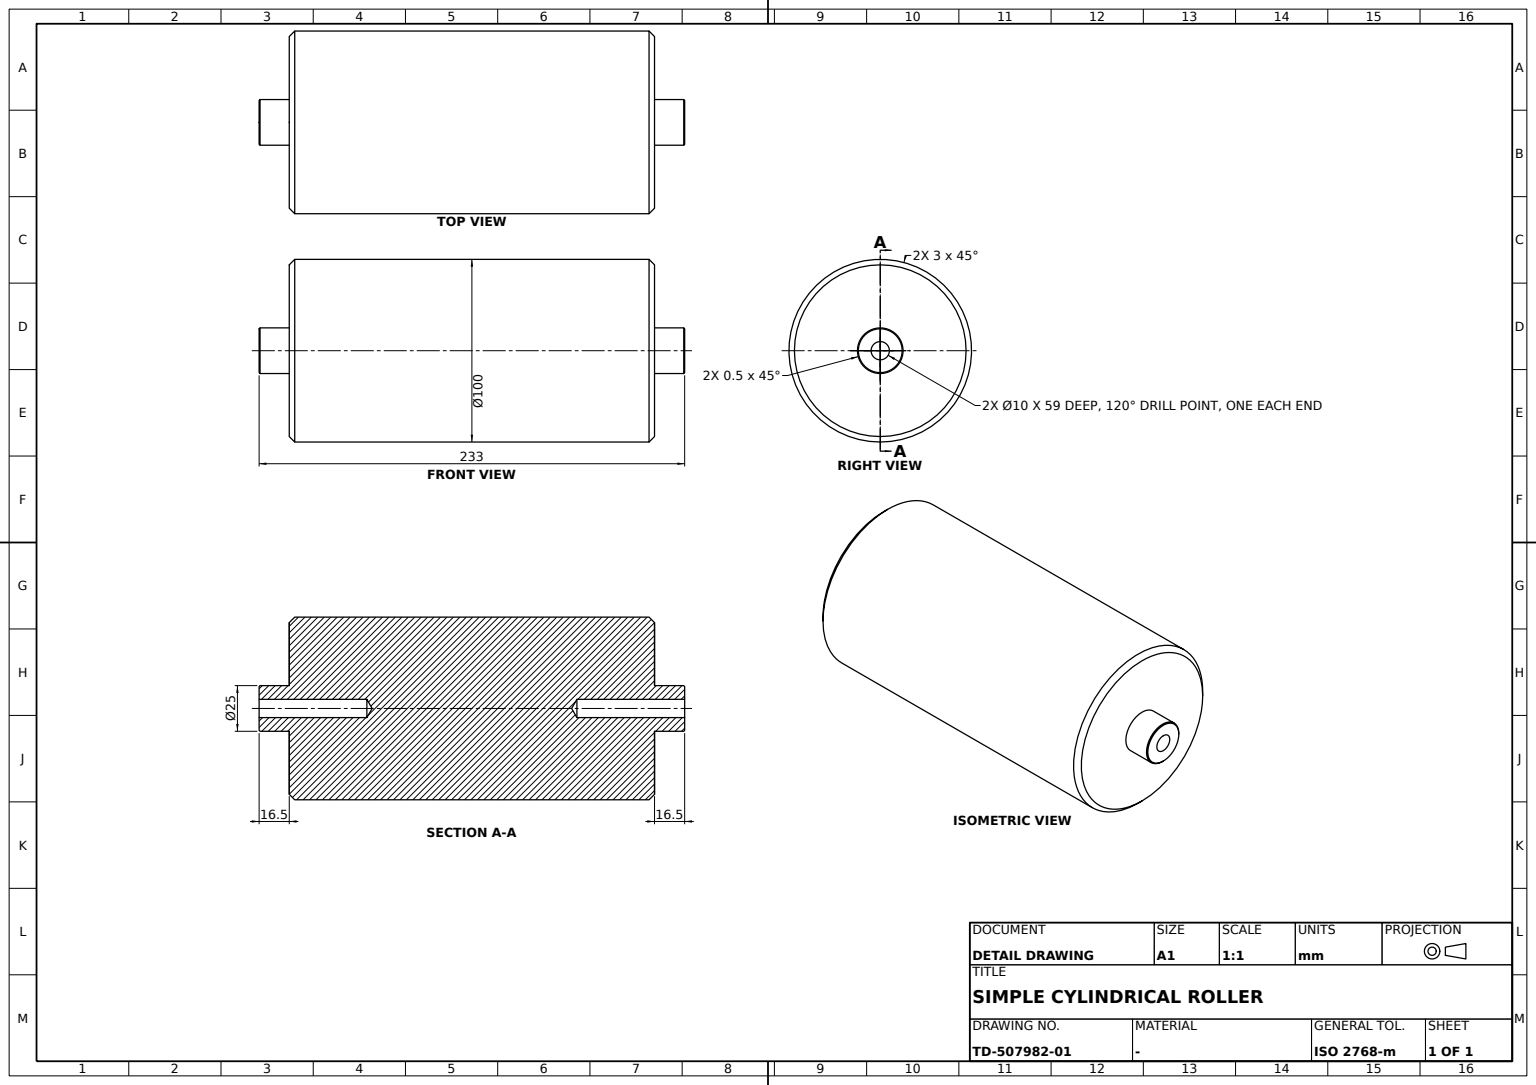
CATIA V5 part; units mm, degrees
sketch "Sketch1" plane through (0, 0, 0) normal (0, 1, 0) x (-1, 0, 0)
  circle A0 centre (0, 0) radius 50
  dimension "radius A0" = 50
extrude "Pad1" add sketch "Sketch1" along normal mid plane 200
chamfer "Chamfer1" distance 3 angle 45 2 edges at (50, 100, 0) (50, -100, 0)
sketch "Sketch2" plane through (0, 100, 0) normal (0, 1, 0) x (-1, 0, 0)
  circle A0 centre (0, 0) radius 12.5
  dimension "radius A0" = 12.5
extrude "Pad2" add sketch "Sketch2" along normal blind 16.5
chamfer "Chamfer2" distance 0.5 angle 45 1 edges at (12.5, 116.5, 0)
mirror "Mirror1" about plane through (0, 0, 0) normal (0, 1, 0) of "Pad2", "Chamfer2"
sketch "Sketch3" plane through (0, 116.5, 0) normal (0, 1, 0) x (1, 0, 0)
  point P0 (0, 0)
  circle A0 centre (0, 0) radius 12.5 construction
  constraint concentricity P0 A0
hole "Hole1" at (0, 116.5, 0) direction (0, -1, 0) diameter 10 depth 50
sketch "Sketch4" plane through (0, 116.5, 0) normal (0, 1, 0) x (1, 0, 0)
  point P0 (0, 0)
  circle A0 centre (0, 0) radius 12 construction
  constraint concentricity P0 A0
hole "Hole2" at (0, 116.5, 0) direction (0, -1, 0) diameter 10 depth 59 tip angle 120
mirror "Mirror2" about plane through (0, 0, 0) normal (0, 1, 0) of "Hole1", "Hole2"
